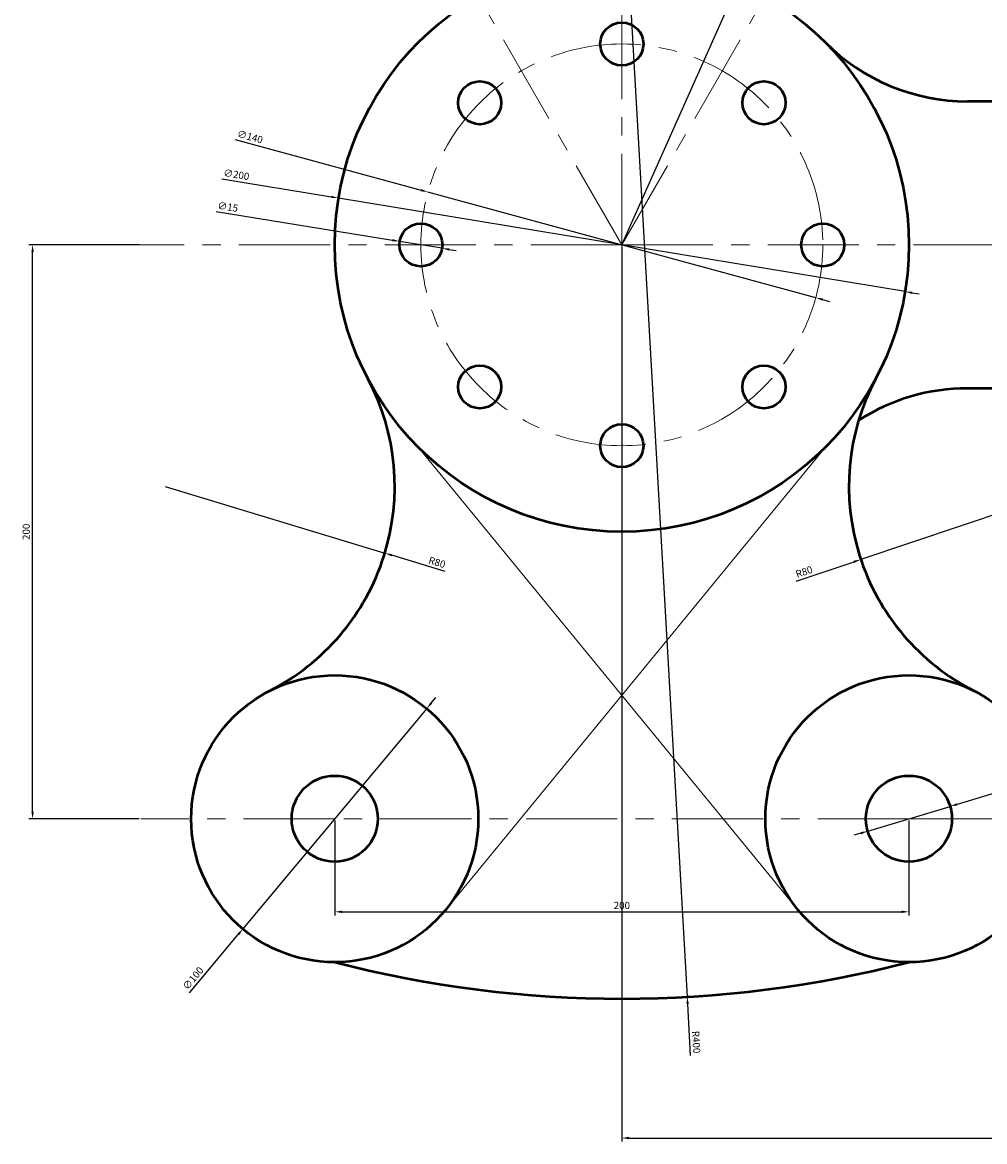
# Model space of a CAD drawing. Units: millimetres. Extents: x 107046 to 107591, y 80056 to 80641.
# Tile 1 of 3: x 107046 to 107381, y 80056 to 80446. Entities that reach past the tile are written whole.
import ezdxf

# ---------------------------------------------------------------- set-up
doc = ezdxf.new("R2010")
doc.units = ezdxf.units.MM
doc.linetypes.add('CENTER', pattern=[50.8, 31.75, -6.35, 6.35, -6.35])
for name, color, linetype, lineweight in [('M-CNTR', 1, 'CENTER', 18), ('M-CONS', 8, 'Continuous', 13), ('M-DIMS', 2, 'Continuous', 25), ('M-OUTL', 7, 'Continuous', 50)]:
    doc.layers.add(name, color=color, linetype=linetype, lineweight=lineweight)
doc.styles.get("Standard").update_dxf_attribs({"font": 'arial.ttf'})
doc.dimstyles.new('ISO-25', dxfattribs={"dimtxt": 2.5, "dimasz": 2.5, "dimexe": 1.25, "dimexo": 0.625, "dimtad": 1, "dimtxsty": 'Standard', "dimcen": 2.5, "dimadec": 0, "dimazin": 0, "dimtfac": 1, "dimtmove": 0, "dimatfit": 3, "dimfxl": 1, "dimarcsym": 0})

# ---------------------------------------------------------------- blocks, each defined once
blk = doc.blocks.new('*D1')
at = {"layer": 'Defpoints', "color": 0, "transparency": 16777216}
for p in [(107049.88, 80368.78), (107087.61, 80368.78), (107087.61, 80168.78)]:
    blk.add_point(p, dxfattribs=at)
at = {"layer": 'M-DIMS', "color": 0, "lineweight": -2, "transparency": 16777216}
for p, q in [((107086.99, 80368.78), (107048.63, 80368.78)), ((107049.88, 80171.28), (107049.88, 80366.28)), ((107086.99, 80168.78), (107048.63, 80168.78))]:
    blk.add_line(p, q, dxfattribs=at)
at = {"layer": 'M-DIMS', "color": 0, "transparency": 16777216}
for points in [[(107049.46, 80366.28), (107050.3, 80366.28), (107049.88, 80368.78)], [(107049.46, 80171.28), (107050.3, 80171.28), (107049.88, 80168.78)]]:
    blk.add_solid(points, dxfattribs=at)
at = {"layer": 'M-DIMS', "color": 0, "transparency": 16777216, "insert": (107047.98, 80268.78), "char_height": 2.5, "attachment_point": 5, "rotation": 90}
blk.add_mtext('200', dxfattribs=at)
blk = doc.blocks.new('*D2')
at = {"layer": 'Defpoints', "color": 0, "transparency": 16777216}
for p in [(107155.14, 80168.78), (107355.14, 80168.78), (107355.14, 80136.36)]:
    blk.add_point(p, dxfattribs=at)
at = {"layer": 'M-DIMS', "color": 0, "lineweight": -2, "transparency": 16777216}
for p, q in [((107155.14, 80168.16), (107155.14, 80135.11)), ((107355.14, 80168.16), (107355.14, 80135.11)), ((107157.64, 80136.36), (107352.64, 80136.36))]:
    blk.add_line(p, q, dxfattribs=at)
at = {"layer": 'M-DIMS', "color": 0, "transparency": 16777216}
for points in [[(107157.64, 80136.77), (107157.64, 80135.94), (107155.14, 80136.36)], [(107352.64, 80136.77), (107352.64, 80135.94), (107355.14, 80136.36)]]:
    blk.add_solid(points, dxfattribs=at)
at = {"layer": 'M-DIMS', "color": 0, "transparency": 16777216, "insert": (107255.14, 80138.26), "char_height": 2.5, "attachment_point": 5}
blk.add_mtext('200', dxfattribs=at)
blk = doc.blocks.new('*D3')
at = {"layer": 'Defpoints', "color": 0, "transparency": 16777216}
for p in [(107255.14, 80368.78), (107555.14, 80368.78), (107555.14, 80057.52)]:
    blk.add_point(p, dxfattribs=at)
at = {"layer": 'M-DIMS', "color": 0, "lineweight": -2, "transparency": 16777216}
for p, q in [((107255.14, 80368.16), (107255.14, 80056.27)), ((107555.14, 80368.16), (107555.14, 80056.27)), ((107257.64, 80057.52), (107552.64, 80057.52))]:
    blk.add_line(p, q, dxfattribs=at)
at = {"layer": 'M-DIMS', "color": 0, "transparency": 16777216}
for points in [[(107257.64, 80057.94), (107257.64, 80057.11), (107255.14, 80057.52)], [(107552.64, 80057.94), (107552.64, 80057.11), (107555.14, 80057.52)]]:
    blk.add_solid(points, dxfattribs=at)
at = {"layer": 'M-DIMS', "color": 0, "transparency": 16777216, "insert": (107405.14, 80059.43), "char_height": 2.5, "attachment_point": 5}
blk.add_mtext('300', dxfattribs=at)
blk = doc.blocks.new('*D12')
at = {"layer": 'Defpoints', "color": 0, "transparency": 16777216}
for p in [(107336.56, 80551.46), (107255.14, 80368.78)]:
    blk.add_point(p, dxfattribs=at)
at = {"layer": 'M-DIMS', "color": 0, "lineweight": -2, "transparency": 16777216}
for p, q in [((107362.18, 80608.95), (107337.58, 80553.74)), ((107255.14, 80368.78), (107336.56, 80551.46))]:
    blk.add_line(p, q, dxfattribs=at)
at = {"layer": 'M-DIMS', "color": 0, "transparency": 16777216}
blk.add_solid([(107337.2, 80553.91), (107337.96, 80553.57), (107336.56, 80551.46)], dxfattribs=at)
at = {"layer": 'M-DIMS', "color": 0, "transparency": 16777216, "insert": (107358.58, 80605.54), "char_height": 2.5, "attachment_point": 5, "rotation": 65.9766}
blk.add_mtext('R200', dxfattribs=at)
blk = doc.blocks.new('*D13')
at = {"layer": 'Defpoints', "color": 0, "transparency": 16777216}
for p in [(107096.05, 80284.58), (107172.6, 80261.34)]:
    blk.add_point(p, dxfattribs=at)
at = {"layer": 'M-DIMS', "color": 0, "lineweight": -2, "transparency": 16777216}
for p, q in [((107096.05, 80284.58), (107172.6, 80261.34)), ((107193.58, 80254.97), (107174.99, 80260.61))]:
    blk.add_line(p, q, dxfattribs=at)
at = {"layer": 'M-DIMS', "color": 0, "transparency": 16777216}
blk.add_solid([(107175.11, 80261.01), (107174.87, 80260.22), (107172.6, 80261.34)], dxfattribs=at)
at = {"layer": 'M-DIMS', "color": 0, "transparency": 16777216, "insert": (107190.68, 80257.84), "char_height": 2.5, "attachment_point": 5, "rotation": 343.1134}
blk.add_mtext('R80', dxfattribs=at)
blk = doc.blocks.new('*D14')
at = {"layer": 'Defpoints', "color": 0, "transparency": 16777216}
for p in [(107414.23, 80284.58), (107338.38, 80259.13)]:
    blk.add_point(p, dxfattribs=at)
at = {"layer": 'M-DIMS', "color": 0, "lineweight": -2, "transparency": 16777216}
for p, q in [((107414.23, 80284.58), (107338.38, 80259.13)), ((107315.92, 80251.6), (107336.01, 80258.34))]:
    blk.add_line(p, q, dxfattribs=at)
at = {"layer": 'M-DIMS', "color": 0, "transparency": 16777216}
blk.add_solid([(107335.88, 80258.73), (107336.14, 80257.94), (107338.38, 80259.13)], dxfattribs=at)
at = {"layer": 'M-DIMS', "color": 0, "transparency": 16777216, "insert": (107318.73, 80254.55), "char_height": 2.5, "attachment_point": 5, "rotation": 18.5455}
blk.add_mtext('R80', dxfattribs=at)
blk = doc.blocks.new('*D15')
at = {"layer": 'Defpoints', "color": 0, "transparency": 16777216}
for p in [(107255.14, 80506.08), (107277.92, 80106.73)]:
    blk.add_point(p, dxfattribs=at)
at = {"layer": 'M-DIMS', "color": 0, "lineweight": -2, "transparency": 16777216}
for p, q in [((107255.14, 80506.08), (107277.92, 80106.73)), ((107279.09, 80086.26), (107278.07, 80104.24))]:
    blk.add_line(p, q, dxfattribs=at)
at = {"layer": 'M-DIMS', "color": 0, "transparency": 16777216}
blk.add_solid([(107278.48, 80104.26), (107277.65, 80104.21), (107277.92, 80106.73)], dxfattribs=at)
at = {"layer": 'M-DIMS', "color": 0, "transparency": 16777216, "insert": (107280.73, 80090.94), "char_height": 2.5, "attachment_point": 5, "rotation": 273.2659}
blk.add_mtext('R400', dxfattribs=at)
blk = doc.blocks.new('*D16')
at = {"layer": 'Defpoints', "color": 0, "transparency": 16777216}
for p in [(107369.5, 80173.1), (107340.77, 80164.47)]:
    blk.add_point(p, dxfattribs=at)
at = {"layer": 'M-DIMS', "color": 0, "lineweight": -2, "transparency": 16777216}
for p, q in [((107434.11, 80192.49), (107371.9, 80173.81)), ((107340.77, 80164.47), (107369.5, 80173.1)), ((107338.38, 80163.75), (107335.98, 80163.03))]:
    blk.add_line(p, q, dxfattribs=at)
at = {"layer": 'M-DIMS', "color": 0, "transparency": 16777216}
for points in [[(107371.78, 80174.21), (107372.02, 80173.42), (107369.5, 80173.1)], [(107338.26, 80164.15), (107338.49, 80163.35), (107340.77, 80164.47)]]:
    blk.add_solid(points, dxfattribs=at)
at = {"layer": 'M-DIMS', "color": 0, "transparency": 16777216, "insert": (107429.93, 80193.29), "char_height": 2.5, "attachment_point": 5, "rotation": 16.7071}
blk.add_mtext('∅30', dxfattribs=at)
blk = doc.blocks.new('*D17')
at = {"layer": 'Defpoints', "color": 0, "transparency": 16777216}
for p in [(107187.16, 80207.19), (107123.12, 80130.38)]:
    blk.add_point(p, dxfattribs=at)
at = {"layer": 'M-DIMS', "color": 0, "lineweight": -2, "transparency": 16777216}
for p, q in [((107188.76, 80209.11), (107190.36, 80211.03)), ((107187.16, 80207.19), (107123.12, 80130.38)), ((107104.51, 80108.07), (107121.52, 80128.46))]:
    blk.add_line(p, q, dxfattribs=at)
at = {"layer": 'M-DIMS', "color": 0, "transparency": 16777216}
for points in [[(107188.44, 80209.37), (107189.08, 80208.84), (107187.16, 80207.19)], [(107121.2, 80128.73), (107121.84, 80128.19), (107123.12, 80130.38)]]:
    blk.add_solid(points, dxfattribs=at)
at = {"layer": 'M-DIMS', "color": 0, "transparency": 16777216, "insert": (107106.04, 80112.97), "char_height": 2.5, "attachment_point": 5, "rotation": 50.1799}
blk.add_mtext('∅100', dxfattribs=at)
blk = doc.blocks.new('*D18')
at = {"layer": 'Defpoints', "color": 0, "transparency": 16777216}
for p in [(107140.14, 80567.97), (107370.14, 80567.97), (107271.77, 80463.13), (107255.14, 80368.78), (107255.14, 80368.78)]:
    blk.add_point(p, dxfattribs=at)
at = {"layer": 'M-DIMS', "color": 0, "lineweight": -2, "transparency": 16777216}
blk.add_arc((107255.14, 80368.78), 95.8, 61.4952, 118.5048, dxfattribs=at)
at = {"layer": 'M-DIMS', "color": 0, "transparency": 16777216}
for points in [[(107209.62, 80452.61), (107209.21, 80453.33), (107207.24, 80451.75)], [(107301.06, 80453.33), (107300.65, 80452.61), (107303.04, 80451.75)]]:
    blk.add_solid(points, dxfattribs=at)
at = {"layer": 'M-DIMS', "color": 0, "transparency": 16777216, "insert": (107255.14, 80466.48), "char_height": 2.5, "attachment_point": 5}
blk.add_mtext('60°', dxfattribs=at)
blk = doc.blocks.new('*D19')
at = {"layer": 'Defpoints', "color": 0, "transparency": 16777216}
for p in [(107177.73, 80369.99), (107192.54, 80367.58)]:
    blk.add_point(p, dxfattribs=at)
at = {"layer": 'M-DIMS', "color": 0, "lineweight": -2, "transparency": 16777216}
for p, q in [((107113.78, 80380.37), (107175.27, 80370.39)), ((107192.54, 80367.58), (107177.73, 80369.99)), ((107195.01, 80367.18), (107197.47, 80366.78))]:
    blk.add_line(p, q, dxfattribs=at)
at = {"layer": 'M-DIMS', "color": 0, "transparency": 16777216}
for points in [[(107175.33, 80370.8), (107175.2, 80369.98), (107177.73, 80369.99)], [(107195.07, 80367.59), (107194.94, 80366.77), (107192.54, 80367.58)]]:
    blk.add_solid(points, dxfattribs=at)
at = {"layer": 'M-DIMS', "color": 0, "transparency": 16777216, "insert": (107117.83, 80381.71), "char_height": 2.5, "attachment_point": 5, "rotation": 350.7737}
blk.add_mtext('∅15', dxfattribs=at)
blk = doc.blocks.new('*D20')
at = {"layer": 'Defpoints', "color": 0, "transparency": 16777216}
for p in [(107156.47, 80385.07), (107353.8, 80352.5)]:
    blk.add_point(p, dxfattribs=at)
at = {"layer": 'M-DIMS', "color": 0, "lineweight": -2, "transparency": 16777216}
for p, q in [((107115.82, 80391.78), (107154.01, 80385.48)), ((107353.8, 80352.5), (107156.47, 80385.07)), ((107356.27, 80352.09), (107358.73, 80351.68))]:
    blk.add_line(p, q, dxfattribs=at)
at = {"layer": 'M-DIMS', "color": 0, "transparency": 16777216}
for points in [[(107154.07, 80385.89), (107153.94, 80385.07), (107156.47, 80385.07)], [(107356.34, 80352.5), (107356.2, 80351.68), (107353.8, 80352.5)]]:
    blk.add_solid(points, dxfattribs=at)
at = {"layer": 'M-DIMS', "color": 0, "transparency": 16777216, "insert": (107120.82, 80392.96), "char_height": 2.5, "attachment_point": 5, "rotation": 350.6259}
blk.add_mtext('∅200', dxfattribs=at)
blk = doc.blocks.new('*D21')
at = {"layer": 'Defpoints', "color": 0, "transparency": 16777216}
for p in [(107187.6, 80387.19), (107322.67, 80350.38)]:
    blk.add_point(p, dxfattribs=at)
at = {"layer": 'M-DIMS', "color": 0, "lineweight": -2, "transparency": 16777216}
for p, q in [((107120.44, 80405.5), (107185.19, 80387.85)), ((107322.67, 80350.38), (107187.6, 80387.19)), ((107325.08, 80349.72), (107327.5, 80349.06))]:
    blk.add_line(p, q, dxfattribs=at)
at = {"layer": 'M-DIMS', "color": 0, "transparency": 16777216}
for points in [[(107185.3, 80388.25), (107185.08, 80387.45), (107187.6, 80387.19)], [(107325.19, 80350.12), (107324.97, 80349.32), (107322.67, 80350.38)]]:
    blk.add_solid(points, dxfattribs=at)
at = {"layer": 'M-DIMS', "color": 0, "transparency": 16777216, "insert": (107125.54, 80406.15), "char_height": 2.5, "attachment_point": 5, "rotation": 344.7533}
blk.add_mtext('∅140', dxfattribs=at)

msp = doc.modelspace()

# ---------------------------------------------------------------- linework, layer by layer
at = {"layer": 'M-CNTR'}
for p, q in [((107255.136, 80368.784), (107255.136, 80641.38)), ((107255.136, 80368.784), (107140.136, 80567.97)), ((107255.136, 80368.784), (107370.136, 80567.97)), ((107255.136, 80368.784), (107075.1, 80368.784)), ((107255.136, 80368.784), (107385.136, 80368.784)), ((107255.136, 80368.784), (107255.136, 80057.245)), ((107155.136, 80168.784), (107087.613, 80168.784)), ((107355.136, 80168.784), (107155.136, 80168.784)), ((107355.136, 80168.784), (107429.433, 80168.784))]:
    msp.add_line(p, q, dxfattribs=at)
msp.add_circle((107255.136, 80368.784), 70, dxfattribs=at)
at = {"layer": 'M-CONS'}
for p, q in [((107184.303, 80298.196), (107316.479, 80137.072)), ((107325.969, 80298.196), (107193.793, 80137.072))]:
    msp.add_line(p, q, dxfattribs=at)
at = {"layer": 'M-OUTL'}
for p, q in [((107535.136, 80418.784), (107375.552, 80418.784)), ((107535.136, 80318.784), (107375.552, 80318.784))]:
    msp.add_line(p, q, dxfattribs=at)
for centre, radius in [((107255.136, 80368.784), 100), ((107255.136, 80438.784), 7.5), ((107205.639, 80418.281), 7.5), ((107304.634, 80418.281), 7.5), ((107185.136, 80368.784), 7.5), ((107325.136, 80368.784), 7.5), ((107205.639, 80319.286), 7.5), ((107304.634, 80319.286), 7.5), ((107255.136, 80298.784), 7.5), ((107155.136, 80168.784), 50), ((107355.136, 80168.784), 50), ((107155.136, 80168.784), 15), ((107355.136, 80168.784), 15)]:
    msp.add_circle(centre, radius, dxfattribs=at)
for centre, radius, start, end in [((107375.552, 80488.784), 70, 224.90087, 270), ((107096.047, 80284.579), 80, 297.03501, 27.89203), ((107414.226, 80284.579), 80, 152.10797, 242.96499), ((107375.552, 80248.784), 70, 90, 122.81909), ((107255.136, 80506.082), 400, 255.52249, 284.47751)]:
    msp.add_arc(centre, radius, start, end, dxfattribs=at)

# ---------------------------------------------------------------- dimensions: what is measured, and where the dimension line sits
at = {"layer": 'M-DIMS'}
for center, mpoint, picture, middle in [((107255.136, 80368.784), (107336.558, 80551.46), '*D12', (107360.32, 80604.77)), ((107255.136, 80506.082), (107277.924, 80106.732), '*D15', (107278.831, 80090.833)), ((107096.047, 80284.579), (107172.597, 80261.34), '*D13', (107190.132, 80256.017)), ((107414.226, 80284.579), (107338.38, 80259.134), '*D14', (107319.339, 80252.746))]:
    dim = msp.add_radius_dim(center=center, mpoint=mpoint, dimstyle='ISO-25', override={"dimclrd": 0, "dimclre": 0, "dimclrt": 0}, dxfattribs=at)
    dim.commit()
    dim.dimension.update_dxf_attribs({"geometry": picture, "text_midpoint": middle, "dimtype": 164})
dim = msp.add_angular_dim_2l(base=(107271.772, 80463.128), line1=((107255.136, 80368.784), (107370.136, 80567.97)), line2=((107255.136, 80368.784), (107140.136, 80567.97)), dimstyle='ISO-25', override={"dimclrd": 0, "dimclre": 0, "dimclrt": 0}, dxfattribs=at)
dim.commit()
dim.dimension.update_dxf_attribs({"geometry": '*D18', "text_midpoint": (107255.136, 80466.485)})
for p1, p2, picture, middle in [((107322.672, 80350.376), (107187.6, 80387.192), '*D21', (107125.02, 80404.25)), ((107353.801, 80352.496), (107156.472, 80385.072), '*D20', (107120.501, 80391.01)), ((107192.539, 80367.581), (107177.733, 80369.986), '*D19', (107117.518, 80379.767)), ((107187.155, 80207.187), (107123.117, 80130.381), '*D17', (107107.552, 80111.712)), ((107340.769, 80164.472), (107369.503, 80173.096), '*D16', (107430.499, 80191.404))]:
    dim = msp.add_diameter_dim_2p(p1=p1, p2=p2, dimstyle='ISO-25', override={"dimclrd": 0, "dimclre": 0, "dimclrt": 0}, dxfattribs=at)
    dim.commit()
    dim.dimension.update_dxf_attribs({"geometry": picture, "text_midpoint": middle, "dimtype": 163})
dim = msp.add_linear_dim(base=(107049.88, 80368.784), p1=(107087.613, 80168.784), p2=(107087.613, 80368.784), angle=90, dimstyle='ISO-25', override={"dimclrd": 0, "dimclre": 0, "dimclrt": 0}, dxfattribs=at)
dim.commit()
dim.dimension.update_dxf_attribs({"geometry": '*D1', "text_midpoint": (107047.979, 80268.784)})
for base, p1, p2, picture, middle in [((107555.136, 80057.524), (107255.136, 80368.784), (107555.136, 80368.784), '*D3', (107405.136, 80059.427)), ((107355.136, 80136.356), (107155.136, 80168.784), (107355.136, 80168.784), '*D2', (107255.136, 80138.257))]:
    dim = msp.add_linear_dim(base=base, p1=p1, p2=p2, dimstyle='ISO-25', override={"dimclrd": 0, "dimclre": 0, "dimclrt": 0}, dxfattribs=at)
    dim.commit()
    dim.dimension.update_dxf_attribs({"geometry": picture, "text_midpoint": middle})

doc.saveas('drawing.dxf')
